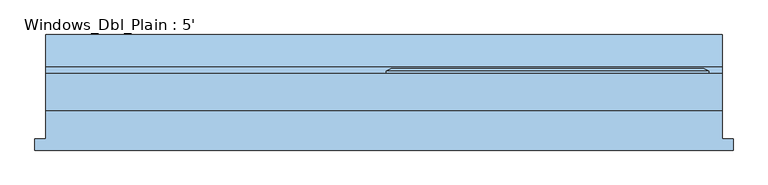
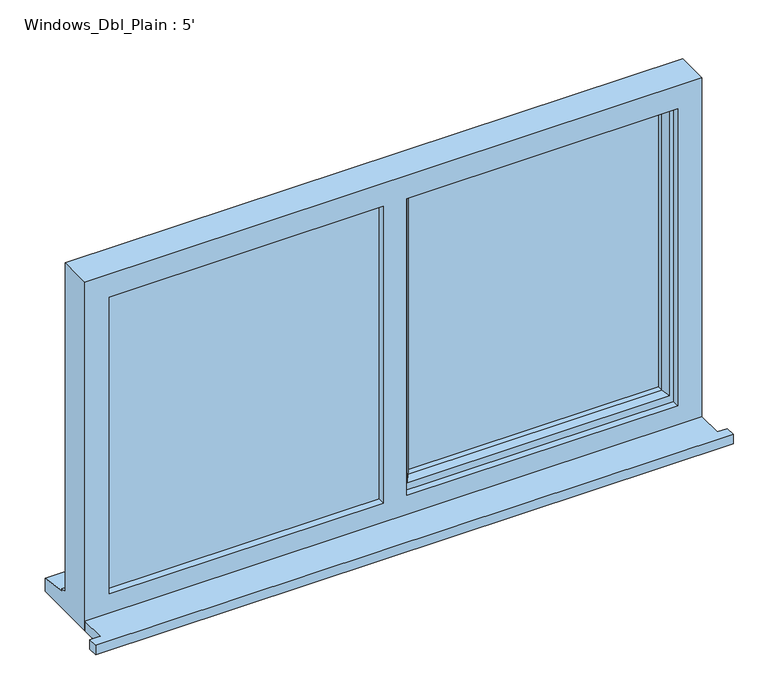
"""IFC4 building model written with IfcOpenShell, lengths in millimetres: window geometry, Windows_Dbl_Plain : 5'."""

from ifc_helpers import new_model, si_unit, frame, origin, place, context, project, spatial, polyline, outline, extrude, faceted_brep, source, transform, mapped, element, save


def windows_dbl_plain_5_c7724a63(model_context):
    return source(origin(), model_context, "Body", "SolidModel", [
        extrude(outline(polyline([(-1072.0, -115.6034322), (-1072.0, -90.6034322), (-1047.0, -90.6034322), (-1047.0, -25.4834322), (477.0, -25.4834322), (477.0, -90.6034322), (502.0, -90.6034322), (502.0, -115.6034322), (-1072.0, -115.6034322)])), frame((0.0, 0.0, 1200.0), z_axis=(0.0, 0.0, 1.0), x_axis=(1.0, 0.0, 0.0)), (0.0, 0.0, 1.0), 25.0),
        faceted_brep([(-280.0, 57.5165678, 2080.0), (-280.0, 63.2900705, 2080.0), (-280.0, 63.2900705, 1253.0), (-280.0, 57.5165678, 1253.0), (-270.0, -7.4834322, 2070.0), (-270.0, 57.5165678, 2070.0), (-270.0, 57.5165678, 1263.0), (-270.0, -7.4834322, 1263.0), (-230.0, 7.0094677, 2030.0), (-240.1480377, -7.4834322, 2040.1480377), (-240.1480377, -7.4834322, 1292.8519623), (-230.0, 7.0094677, 1303.0), (-230.0, 21.5165678, 2030.0), (-230.0, 21.5165678, 1303.0), (-240.0, 45.5165678, 2040.0), (-240.0, 21.5165678, 2040.0), (-240.0, 21.5165678, 1293.0), (-240.0, 45.5165678, 1293.0), (-230.0, 63.2900705, 2030.0), (-230.0, 45.5165678, 2030.0), (-230.0, 45.5165678, 1303.0), (-230.0, 63.2900705, 1303.0), (-247.4457548, 69.0635732, 2047.4457548), (-247.4457548, 69.0635732, 1285.5542452), (-269.2153903, 69.0635732, 2069.2153903), (-269.2153903, 69.0635732, 1263.7846097), (447.0, 63.2900705, 1253.0), (447.0, 57.5165678, 1253.0), (437.0, 57.5165678, 1263.0), (437.0, -7.4834322, 1263.0), (407.1480377, -7.4834322, 1292.8519623), (397.0, 7.0094677, 1303.0), (397.0, 21.5165678, 1303.0), (407.0, 21.5165678, 1293.0), (407.0, 45.5165678, 1293.0), (397.0, 45.5165678, 1303.0), (397.0, 63.2900705, 1303.0), (414.4457548, 69.0635732, 1285.5542452), (436.2153903, 69.0635732, 1263.7846097), (447.0, 63.2900705, 2080.0), (447.0, 57.5165678, 2080.0), (437.0, 57.5165678, 2070.0), (437.0, -7.4834322, 2070.0), (407.1480377, -7.4834322, 2040.1480377), (397.0, 7.0094677, 2030.0), (397.0, 21.5165678, 2030.0), (407.0, 21.5165678, 2040.0), (407.0, 45.5165678, 2040.0), (397.0, 45.5165678, 2030.0), (397.0, 63.2900705, 2030.0), (414.4457548, 69.0635732, 2047.4457548), (436.2153903, 69.0635732, 2069.2153903)], [[[0, 1, 2, 3]], [[4, 5, 6, 7]], [[8, 9, 10, 11]], [[12, 8, 11, 13]], [[14, 15, 16, 17]], [[18, 19, 20, 21]], [[22, 18, 21, 23]], [[1, 24, 25, 2]], [[3, 2, 26, 27]], [[7, 6, 28, 29]], [[11, 10, 30, 31]], [[13, 11, 31, 32]], [[17, 16, 33, 34]], [[21, 20, 35, 36]], [[23, 21, 36, 37]], [[2, 25, 38, 26]], [[27, 26, 39, 40]], [[29, 28, 41, 42]], [[31, 30, 43, 44]], [[32, 31, 44, 45]], [[34, 33, 46, 47]], [[36, 35, 48, 49]], [[37, 36, 49, 50]], [[26, 38, 51, 39]], [[40, 39, 1, 0]], [[3, 27, 40, 0], [5, 41, 28, 6]], [[42, 41, 5, 4]], [[7, 29, 42, 4], [9, 43, 30, 10]], [[44, 43, 9, 8]], [[45, 44, 8, 12]], [[15, 46, 33, 16], [13, 32, 45, 12]], [[47, 46, 15, 14]], [[17, 34, 47, 14], [19, 48, 35, 20]], [[49, 48, 19, 18]], [[50, 49, 18, 22]], [[24, 51, 38, 25], [23, 37, 50, 22]], [[39, 51, 24, 1]]]),
        extrude(outline(polyline([(2050.0, -310.0), (2070.0, -310.0), (2070.0, -1007.0), (1263.0, -1007.0), (1263.0, -310.0), (1283.0, -310.0), (1283.0, -987.0), (2050.0, -987.0), (2050.0, -310.0)])), frame((0.0, 16.5165678, 0.0), z_axis=(0.0, 1.0, 0.0), x_axis=(0.0, 0.0, 1.0)), (0.0, 0.0, 1.0), 41.0),
        faceted_brep([(477.0, -25.4834322, 2110.0), (-1047.0, -25.4834322, 2110.0), (-1047.0, -25.4834322, 1200.0), (477.0, -25.4834322, 1200.0), (417.0, -25.4834322, 2050.0), (417.0, -25.4834322, 1275.0), (-252.0, -25.4834322, 1275.0), (-252.0, -25.4834322, 2050.0), (-310.0, -25.4834322, 2050.0), (-310.0, -25.4834322, 1275.0), (-987.0, -25.4834322, 1275.0), (-987.0, -25.4834322, 2050.0), (-1047.0, 57.5165678, 2110.0), (-1047.0, 57.5165678, 1251.0), (-1047.0, 72.5165678, 1249.68767), (-1047.0, 72.5165678, 1244.7449676), (-1047.0, 145.0165678, 1233.8088847), (-1047.0, 145.0165678, 1200.0), (477.0, 57.5165678, 2110.0), (477.0, 57.5165678, 1251.0), (-1007.0, 57.5165678, 2070.0), (-1007.0, 57.5165678, 1263.0), (-310.0, 57.5165678, 1263.0), (-310.0, 57.5165678, 2070.0), (-270.0, 57.5165678, 2070.0), (-270.0, 57.5165678, 1263.0), (437.0, 57.5165678, 1263.0), (437.0, 57.5165678, 2070.0), (-1007.0, -7.4834322, 2070.0), (-1007.0, -7.4834322, 1263.0), (-300.0, -7.4834322, 2070.0), (-300.0, -7.4834322, 1263.0), (-310.0, -7.4834322, 2050.0), (-987.0, -7.4834322, 2050.0), (-987.0, -7.4834322, 1275.0), (-310.0, -7.4834322, 1275.0), (-270.0, -7.4834322, 2070.0), (437.0, -7.4834322, 2070.0), (437.0, -7.4834322, 1263.0), (-270.0, -7.4834322, 1263.0), (417.0, -7.4834322, 2050.0), (-252.0, -7.4834322, 2050.0), (-252.0, -7.4834322, 1275.0), (417.0, -7.4834322, 1275.0), (-310.0, 16.5165678, 2070.0), (-300.0, 16.5165678, 2070.0), (477.0, 145.0165678, 1200.0), (477.0, 145.0165678, 1233.8088847), (477.0, 72.5165678, 1244.7449676), (477.0, 72.5165678, 1249.68767), (-300.0, 16.5165678, 1263.0), (-310.0, 16.5165678, 1263.0)], [[[0, 1, 2, 3], [4, 5, 6, 7], [8, 9, 10, 11]], [[2, 1, 12, 13, 14, 15, 16, 17]], [[13, 12, 18, 19], [20, 21, 22, 23], [24, 25, 26, 27]], [[21, 20, 28, 29]], [[28, 30, 31, 29], [32, 33, 34, 35]], [[36, 37, 38, 39], [40, 41, 42, 43]], [[33, 11, 10, 34]], [[1, 0, 18, 12]], [[28, 20, 23, 44, 45, 30]], [[27, 37, 36, 24]], [[11, 33, 32, 8]], [[40, 4, 7, 41]], [[19, 18, 0, 3, 46, 47, 48, 49]], [[27, 26, 38, 37]], [[4, 40, 43, 5]], [[45, 50, 31, 30]], [[50, 45, 44, 51]], [[51, 44, 23, 22]], [[25, 24, 36, 39]], [[41, 7, 6, 42]], [[8, 32, 35, 9]], [[46, 3, 2, 17]], [[47, 46, 17, 16]], [[48, 47, 16, 15]], [[49, 48, 15, 14]], [[19, 49, 14, 13]], [[22, 21, 29, 31, 50, 51]], [[26, 25, 39, 38]], [[6, 5, 43, 42]], [[35, 34, 10, 9]]]),
        extrude(outline(polyline([(-1007.0, 16.5165678), (-300.0, 16.5165678), (-300.0, -7.4834322), (-1007.0, -7.4834322), (-1007.0, 16.5165678)])), frame((0.0, 0.0, 1263.0), z_axis=(0.0, 0.0, 1.0), x_axis=(1.0, 0.0, 0.0)), (0.0, 0.0, 1.0), 807.0),
        extrude(outline(polyline([(407.0, 21.5165678), (-240.0, 21.5165678), (-240.0, 45.5165678), (407.0, 45.5165678), (407.0, 21.5165678)])), frame((0.0, 0.0, 1293.0), z_axis=(0.0, 0.0, 1.0), x_axis=(1.0, 0.0, 0.0)), (0.0, 0.0, 1.0), 747.0),
    ])


if __name__ == "__main__":
    model = new_model("IFC4")
    model_context = context("Model", 3, world=origin())
    ifc_project = project(units=[si_unit("LENGTHUNIT", "METRE", prefix="MILLI")], contexts=[model_context])
    site = spatial("IfcSite", under=ifc_project)
    building = spatial("IfcBuilding", under=site)
    placement = place(None, origin())
    windows_dbl_plain_5_shape = windows_dbl_plain_5_c7724a63(model_context)
    element("IfcWindow", 1, ObjectType="Windows_Dbl_Plain : 5'", at=placement, inside=building, context=model_context, shape_type="MappedRepresentation", body=[
        mapped(windows_dbl_plain_5_shape, transform((0.0, 0.0, 0.0), x_axis=(1.0, 0.0, 0.0), y_axis=(0.0, 1.0, 0.0), z_axis=(0.0, 0.0, 1.0))),
    ])
    save(model, "model.ifc")

# Revit data of these elements
# Type "Windows_Dbl_Plain : 5'"
#   Type Mark = "58"
#   Operation = "DoublePanelVertical"
#   Construction Type Id = "GSP4R"
#   Manufacturer = "Revit"
#   Keynote = "L10"
#   Analytic Construction = "1/8 in Pilkington single glazing"
#   Wrap Layers (Ext) from Ext = 0.336286 ft
#   Wrap Layers (Int) from Ext = 0.582349 ft
#   Window Board Projection = 0.082021 ft
#   Window Board Extension = 0.082021 ft
#   Visual Light Transmittance = 0.9
#   Solar Heat Gain Coefficient = 0.78
#   Rough Width = 5.0 ft
#   Rough Height = 2.985564 ft
#   Height = 2.985564 ft
#   Width = 5.0 ft
#   Heat Transfer Coefficient (U) = 3.6886 W/(m²·K)
#   Glazing Thickness = 0.07874 ft
#   FrameOffset - External = 0.164042 ft
#   Frame Depth = 0.213255 ft
#   Default Head Height = 6.922572 ft
#   Cill Depth = 0.287073 ft
#   Cavity Closer Width = 0.164042 ft
#   Cavity Closer Offset from Ext = 0.336286 ft
#   Cavity Closer Depth = 0.278871 ft
#   Vis - Cavity Closers = yes
#   Define Thermal Properties by = 1
#   Material Trim = Window Frame
#   Material Glass = Glass
#   Material Frame = Window Frame
#   Wall Closure = (empty or 0)
# Element 1 (IfcWindow, "Windows_Dbl_Plain : 5'")
#   Materials on its faces: "Window Frame", "Glass"
# Materials
#   "Window Frame": colour RGB 249 249 249, transparency 0, Keynote = "L10", Cost = 0
#   "Glass": class "Glass", colour RGB 0 128 192, transparency 0.9, Description = "Soda Lime Glass", Cost = 0
